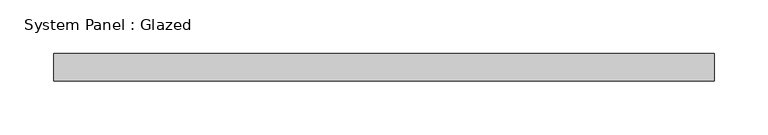
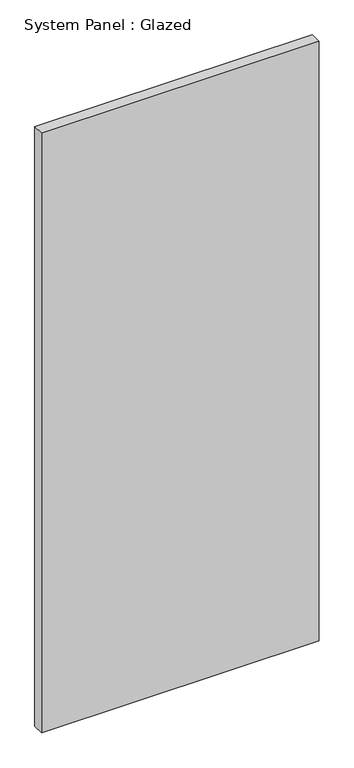
"""IFC4 building model written with IfcOpenShell, lengths in millimetres: plate geometry, System Panel : Glazed."""

from ifc_helpers import new_model, si_unit, origin, origin_with_axes, place, context, project, spatial, polyline, outline, extrude, source, transform, mapped, element, save


def system_panel_glazed_db10fc3c(model_context):
    return source(origin(), model_context, "Body", "SweptSolid", [
        extrude(outline(polyline([(306.8664477, 19.05), (-306.8664477, 19.05), (-306.8664477, 44.45), (306.8664477, 44.45), (306.8664477, 19.05)])), origin_with_axes(), (0.0, 0.0, 1.0), 1401.6649662),
    ])


if __name__ == "__main__":
    model = new_model("IFC4")
    model_context = context("Model", 3, world=origin())
    ifc_project = project(units=[si_unit("LENGTHUNIT", "METRE", prefix="MILLI")], contexts=[model_context])
    site = spatial("IfcSite", under=ifc_project)
    building = spatial("IfcBuilding", under=site)
    placement = place(None, origin())
    system_panel_glazed_shape = system_panel_glazed_db10fc3c(model_context)
    element("IfcPlate", 1, ObjectType="System Panel : Glazed", at=placement, inside=building, context=model_context, shape_type="MappedRepresentation", body=[
        mapped(system_panel_glazed_shape, transform((0.0, 0.0, 0.0), x_axis=(1.0, 0.0, 0.0), y_axis=(0.0, 1.0, 0.0), z_axis=(0.0, 0.0, 1.0))),
    ])
    save(model, "model.ifc")

# Revit data of these elements
# Type "System Panel : Glazed"
#   Construction Type Id = "GSP4R"
#   Analytic Construction = "1/8 in Pilkington single glazing"
#   Visual Light Transmittance = 0.9
#   Solar Heat Gain Coefficient = 0.86
#   Heat Transfer Coefficient (U) = 1.18115 BTU/(h·ft²·°F)
#   Define Thermal Properties by = 1
# Element 1 (IfcPlate, "System Panel : Glazed")
#   Materials on its faces: "Glass"
# Materials
#   "Glass": class "Glass", colour RGB 0 128 192, transparency 0.75, Description = "Soda Lime Glass", Cost = 0
